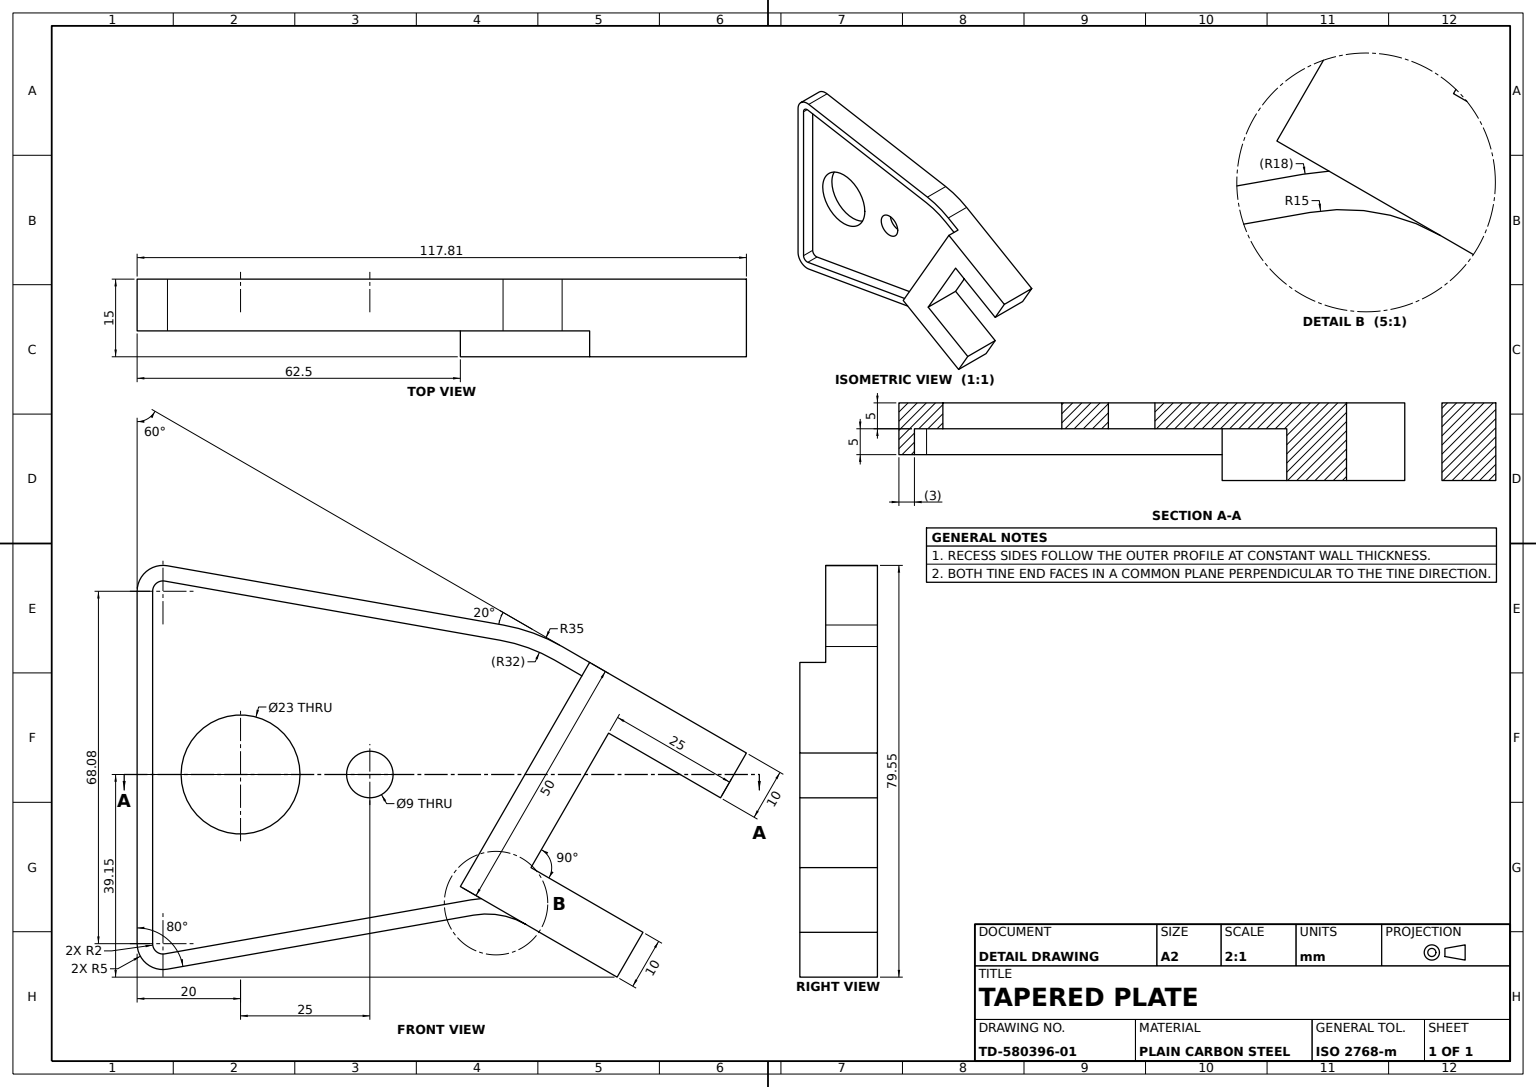
SolidWorks part; units mm, degrees
material "Plain Carbon Steel"
ref_plane "Front Plane" through (0, 0, 0) normal (0, 0, 1) x (1, 0, 0)
ref_plane "Top Plane" through (0, 0, 0) normal (0, 1, 0) x (1, 0, 0)
ref_plane "Right Plane" through (0, 0, 0) normal (1, 0, 0) x (0, 0, -1)
sketch "Base Plate Profile Sketch" plane through (0, 0, 0) normal (0, 1, 0) x (1, 0, 0)
  line L0 (-28.8799, 70.7571) -> (-40.3215, 5.8682)
  line L1 (-35.3975, 0) -> (32.685, 0)
  line L2 (37.609, 5.8682) -> (27.174, 65.0481)
  line L3 (0, 75) -> (0, -118.209) construction
  line L4 (-4.1506, 117.8109) -> (-24.7225, 82.1794)
  line L5 (-14.8559, 49.2689) -> (17.3205, 105) construction
  line L6 (-4.1506, 117.8109) -> (4.5096, 112.8109)
  line L7 (-21.6506, 87.5) -> (21.6506, 62.5)
  line L8 (21.6506, 62.5) -> (39.1506, 92.8109)
  line L9 (-7.9904, 91.1603) -> (17.9904, 76.1603)
  line L10 (4.5096, 112.8109) -> (-7.9904, 91.1603)
  line L11 (17.9904, 76.1603) -> (30.4904, 97.8109)
  line L12 (30.4904, 97.8109) -> (39.1506, 92.8109)
  line L13 (4.5096, 112.8109) -> (-19.1479, 71.8348) construction
  line L14 (-4.1506, 117.8109) -> (-27.8082, 76.8348) construction
  line L15 (-16.6506, 96.1603) -> (26.6506, 71.1603) construction
  line L16 (12.9904, 67.5) -> (30.4904, 97.8109) construction
  line L17 (21.6506, 62.5) -> (39.1506, 92.8109) construction
  line L18 (-19.0526, 86) -> (-22.1244, 80.6794)
  line L19 (-25.9254, 70.2362) -> (-37.3671, 5.3473)
  line L20 (-35.3975, 3) -> (32.685, 3)
  line L21 (34.6546, 5.3473) -> (24.2196, 64.5272)
  line L23 (-1.5526, 116.3109) -> (-22.1244, 80.6794) construction
  arc A0 (32.685, 0) -> (37.609, 5.8682) centre (32.685, 5) ccw
  arc A1 (-40.3215, 5.8682) -> (-35.3975, 0) centre (-35.3975, 5) ccw
  circle A2 centre (0, 20) radius 11.5
  circle A3 centre (0, 45) radius 4.5
  arc A5 (-28.8799, 70.7571) -> (-24.7225, 82.1794) centre (5.5884, 64.6794) cw
  arc A6 (28.9558, 75.1528) -> (27.174, 65.0481) centre (41.9461, 67.6528) ccw
  arc A7 (-25.9254, 70.2362) -> (-22.1244, 80.6794) centre (5.5884, 64.6794) cw
  arc A8 (-37.3671, 5.3473) -> (-35.3975, 3) centre (-35.3975, 5) ccw
  arc A9 (32.685, 3) -> (34.6546, 5.3473) centre (32.685, 5) ccw
  arc A10 (23.9808, 66.536) -> (24.2196, 64.5272) centre (41.9461, 67.6528) ccw
  arc A12 (26.3577, 76.6528) -> (24.2196, 64.5272) centre (41.9461, 67.6528) ccw construction
  point P8 (38.6438, 0)
  point P11 (-41.3562, 0)
  dimension "D3" = 5
  dimension "D6" = 9
  dimension "D7" = 23
  dimension "D18" = 35
  dimension "D19" = 15
  dimension "D1" = 80
  dimension "D2" = 20
  dimension "D4" = 10
  dimension "D5" = 60
  dimension "D8" = 25
  dimension "D9" = 20
  dimension "D10" = 25
  dimension "D11" = 75
  dimension "D12" = 105
  dimension "D13" = 50
  dimension "D14" = 35
  dimension "D21" = 38.6438
  dimension "D15" = 10
  dimension "D16" = 10
  dimension "D17" = 10
  dimension "D20" = 3
extrude "Base Plate" add sketch "Base Plate Profile Sketch" along normal blind 10 contours L8 A10 L21 A9 L20 A8 L19 A7 L18 L7 L4 A5 L0 A1 L1 A0 L2 A6
sketch "Rim Wall Sketch" plane through (0, 0, 0) normal (0, 1, 0) x (1, 0, 0)
  line L0 (-4.1506, 117.8109) -> (-24.7225, 82.1794) construction
  line L1 (21.6506, 62.5) -> (39.1506, 92.8109) construction
  line L2 (-21.6506, 87.5) -> (21.6506, 62.5) construction
  line L3 (34.6546, 5.3473) -> (24.2196, 64.5272) construction
  line L4 (-35.3975, 3) -> (32.685, 3) construction
  line L5 (-25.9254, 70.2362) -> (-37.3671, 5.3473) construction
  line L6 (-19.0526, 86) -> (-22.1244, 80.6794) construction
  line L7 (-4.1506, 117.8109) -> (-24.7225, 82.1794)
  line L8 (21.6506, 62.5) -> (39.1506, 92.8109)
  line L9 (-21.6506, 87.5) -> (21.6506, 62.5)
  line L10 (34.6546, 5.3473) -> (24.2196, 64.5272)
  line L11 (-35.3975, 3) -> (32.685, 3)
  line L12 (-25.9254, 70.2362) -> (-37.3671, 5.3473)
  line L13 (-19.0526, 86) -> (-22.1244, 80.6794)
  line L14 (-4.1506, 117.8109) -> (4.5096, 112.8109) construction
  line L15 (30.4904, 97.8109) -> (39.1506, 92.8109) construction
  line L16 (17.9904, 76.1603) -> (30.4904, 97.8109) construction
  line L17 (-7.9904, 91.1603) -> (17.9904, 76.1603) construction
  line L18 (4.5096, 112.8109) -> (-7.9904, 91.1603) construction
  line L19 (-28.8799, 70.7571) -> (-40.3215, 5.8682) construction
  line L20 (37.609, 5.8682) -> (27.174, 65.0481) construction
  line L21 (-35.3975, 0) -> (32.685, 0) construction
  line L22 (-4.1506, 117.8109) -> (4.5096, 112.8109)
  line L23 (30.4904, 97.8109) -> (39.1506, 92.8109)
  line L24 (17.9904, 76.1603) -> (30.4904, 97.8109)
  line L25 (-7.9904, 91.1603) -> (17.9904, 76.1603)
  line L26 (4.5096, 112.8109) -> (-7.9904, 91.1603)
  line L27 (-28.8799, 70.7571) -> (-40.3215, 5.8682)
  line L28 (37.609, 5.8682) -> (27.174, 65.0481)
  line L29 (-35.3975, 0) -> (32.685, 0)
  arc A0 (32.685, 3) -> (34.6546, 5.3473) centre (32.685, 5) ccw construction
  arc A1 (-37.3671, 5.3473) -> (-35.3975, 3) centre (-35.3975, 5) ccw construction
  circle A2 centre (0, 20) radius 11.5 construction
  circle A3 centre (0, 45) radius 4.5 construction
  arc A4 (-22.1244, 80.6794) -> (-25.9254, 70.2362) centre (5.5884, 64.6794) ccw construction
  arc A5 (32.685, 3) -> (34.6546, 5.3473) centre (32.685, 5) ccw
  arc A6 (-37.3671, 5.3473) -> (-35.3975, 3) centre (-35.3975, 5) ccw
  circle A7 centre (0, 20) radius 11.5
  circle A8 centre (0, 45) radius 4.5
  arc A9 (-22.1244, 80.6794) -> (-25.9254, 70.2362) centre (5.5884, 64.6794) ccw
  arc A10 (28.9558, 75.1528) -> (27.174, 65.0481) centre (41.9461, 67.6528) ccw construction
  arc A11 (23.9808, 66.536) -> (24.2196, 64.5272) centre (41.9461, 67.6528) ccw construction
  arc A12 (-24.7225, 82.1794) -> (-28.8799, 70.7571) centre (5.5884, 64.6794) ccw construction
  arc A13 (-40.3215, 5.8682) -> (-35.3975, 0) centre (-35.3975, 5) ccw construction
  arc A14 (32.685, 0) -> (37.609, 5.8682) centre (32.685, 5) ccw construction
  arc A15 (28.9558, 75.1528) -> (27.174, 65.0481) centre (41.9461, 67.6528) ccw
  arc A16 (23.9808, 66.536) -> (24.2196, 64.5272) centre (41.9461, 67.6528) ccw
  arc A17 (-24.7225, 82.1794) -> (-28.8799, 70.7571) centre (5.5884, 64.6794) ccw
  arc A18 (-40.3215, 5.8682) -> (-35.3975, 0) centre (-35.3975, 5) ccw
  arc A19 (32.685, 0) -> (37.609, 5.8682) centre (32.685, 5) ccw
extrude "Rim Wall" add sketch "Rim Wall Sketch" along normal blind 5 contours A16 L8 L9 L13 A9 L12 A6 L11 A5 L10 A8 A7
sketch "Fork Block Sketch" plane through (0, 0, 0) normal (0, 1, 0) x (1, 0, 0)
  line L0 (30.4904, 97.8109) -> (39.1506, 92.8109) construction
  line L1 (17.9904, 76.1603) -> (30.4904, 97.8109) construction
  line L2 (21.6506, 62.5) -> (39.1506, 92.8109) construction
  line L3 (-21.6506, 87.5) -> (21.6506, 62.5) construction
  line L4 (-7.9904, 91.1603) -> (17.9904, 76.1603) construction
  line L5 (-4.1506, 117.8109) -> (-24.7225, 82.1794) construction
  line L6 (-4.1506, 117.8109) -> (4.5096, 112.8109) construction
  line L7 (4.5096, 112.8109) -> (-7.9904, 91.1603) construction
  line L8 (30.4904, 97.8109) -> (39.1506, 92.8109)
  line L9 (17.9904, 76.1603) -> (30.4904, 97.8109)
  line L10 (21.6506, 62.5) -> (39.1506, 92.8109)
  line L11 (-21.6506, 87.5) -> (21.6506, 62.5)
  line L12 (-7.9904, 91.1603) -> (17.9904, 76.1603)
  line L13 (-4.1506, 117.8109) -> (-24.7225, 82.1794)
  line L14 (-4.1506, 117.8109) -> (4.5096, 112.8109)
  line L15 (4.5096, 112.8109) -> (-7.9904, 91.1603)
extrude "Fork Block" add sketch "Fork Block Sketch" along normal blind 15 contours L15 L14 L13 L11 L10 L8 L9 L12
